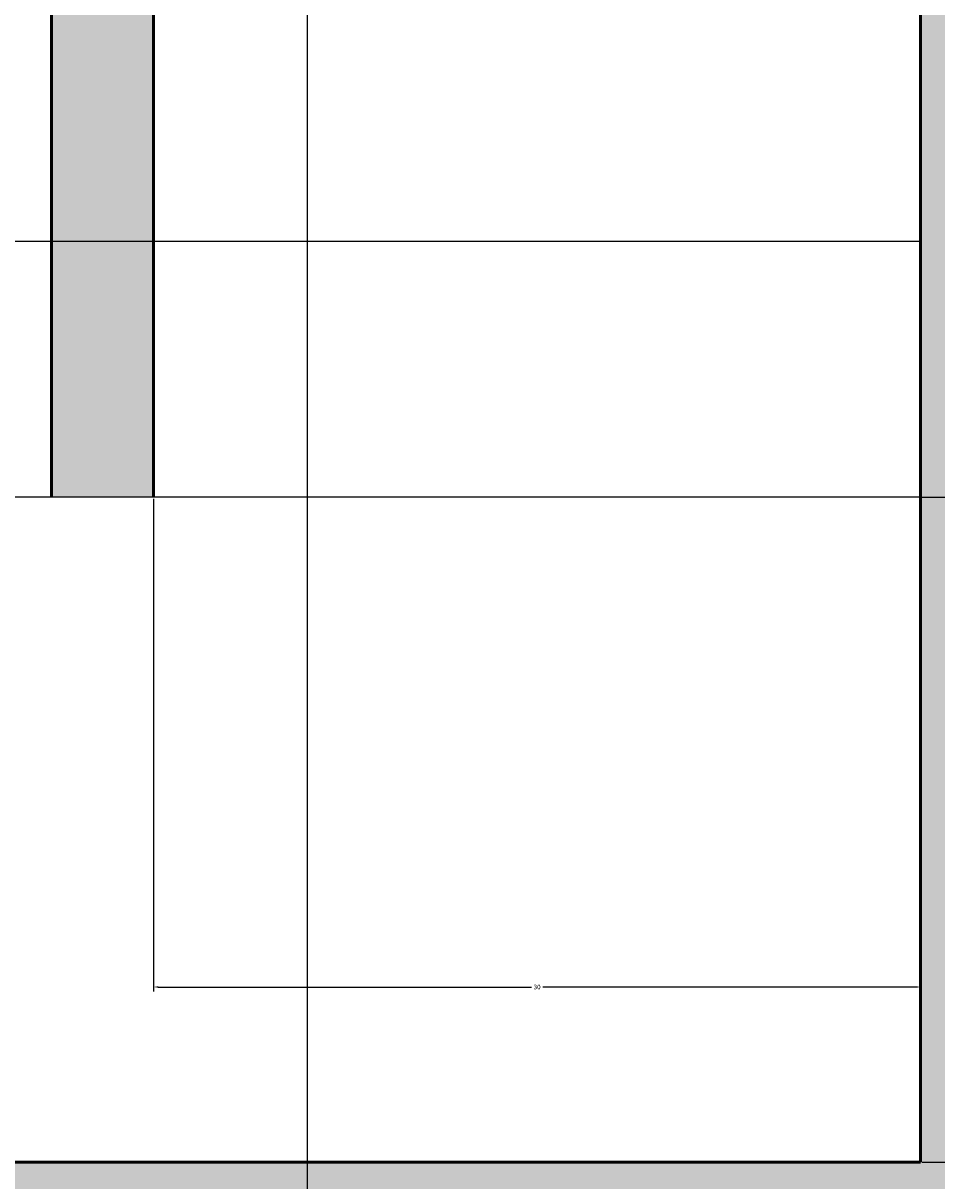
# Model space of a CAD drawing. Units: inches. Extents: x 2307 to 2544, y 2171 to 2540.
# Tile 11 of 52: x 2481 to 2516, y 2199 to 2244. Entities that reach past the tile are written whole.
import ezdxf

# ---------------------------------------------------------------- set-up
doc = ezdxf.new("R2010")
doc.units = ezdxf.units.IN
for name, color, linetype, lineweight in [('A-ANNO-DIMS', 2, 'Continuous', 18), ('A-FLOR-STRS', 7, 'Continuous', 25), ('A-WALL', 7, 'Continuous', 50)]:
    doc.layers.add(name, color=color, linetype=linetype, lineweight=lineweight)
doc.layers.add('A-WALL-PATT', color=18, linetype='Continuous', lineweight=13, true_color=0x000000)
doc.styles.get("Standard").update_dxf_attribs({"font": 'arial.ttf'})
doc.dimstyles.get("Standard").update_dxf_attribs({"dimtxt": 0.18, "dimasz": 0.18, "dimexe": 0.18, "dimexo": 0.0625, "dimgap": 0.09, "dimtad": 0, "dimtih": 1, "dimtoh": 1, "dimdec": 4, "dimzin": 0, "dimdsep": 46, "dimtxsty": 'Standard', "dimcen": 0.09, "dimadec": 0, "dimazin": 0, "dimtfac": 1, "dimtdec": 4, "dimtofl": 0, "dimtmove": 0, "dimatfit": 3, "dimfxl": 1, "dimtolj": 1, "dimtzin": 0, "dimarcsym": 0})

# ---------------------------------------------------------------- blocks, each defined once
blk = doc.blocks.new('*D54')
at = {"layer": 'A-ANNO-DIMS', "color": 0, "lineweight": -2, "transparency": 16777216}
for p, q in [((2461.696, 2435.447), (2461.696, 2171.18)), ((2491.696, 2435.447), (2491.696, 2171.18)), ((2461.876, 2171.36), (2476.477, 2171.36)), ((2491.516, 2171.36), (2476.914, 2171.36))]:
    blk.add_line(p, q, dxfattribs=at)
at = {"layer": 'A-ANNO-DIMS', "color": 0, "transparency": 16777216}
for points in [[(2461.876, 2171.39), (2461.876, 2171.33), (2461.696, 2171.36)], [(2491.516, 2171.39), (2491.516, 2171.33), (2491.696, 2171.36)]]:
    blk.add_solid(points, dxfattribs=at)
at = {"layer": 'Defpoints', "color": 0, "transparency": 16777216}
for p in [(2461.696, 2435.51), (2491.696, 2435.51), (2491.696, 2171.36)]:
    blk.add_point(p, dxfattribs=at)
at = {"layer": 'A-ANNO-DIMS', "color": 0, "transparency": 16777216, "insert": (2476.696, 2171.36), "char_height": 0.18, "attachment_point": 5}
blk.add_mtext('\\A1;30', dxfattribs=at)
blk = doc.blocks.new('*D55')
at = {"layer": 'A-ANNO-DIMS', "color": 0, "lineweight": -2, "transparency": 16777216}
for p, q in [((2485.696, 2225.447), (2485.696, 2206.18)), ((2515.696, 2225.447), (2515.696, 2206.18)), ((2485.876, 2206.36), (2500.477, 2206.36)), ((2515.516, 2206.36), (2500.914, 2206.36))]:
    blk.add_line(p, q, dxfattribs=at)
at = {"layer": 'A-ANNO-DIMS', "color": 0, "transparency": 16777216}
for points in [[(2485.876, 2206.39), (2485.876, 2206.33), (2485.696, 2206.36)], [(2515.516, 2206.39), (2515.516, 2206.33), (2515.696, 2206.36)]]:
    blk.add_solid(points, dxfattribs=at)
at = {"layer": 'Defpoints', "color": 0, "transparency": 16777216}
for p in [(2485.696, 2225.51), (2515.696, 2225.51), (2485.696, 2206.36)]:
    blk.add_point(p, dxfattribs=at)
at = {"layer": 'A-ANNO-DIMS', "color": 0, "transparency": 16777216, "insert": (2500.696, 2206.36), "char_height": 0.18, "attachment_point": 5}
blk.add_mtext('\\A1;30', dxfattribs=at)
blk = doc.blocks.new('*D56')
at = {"layer": 'A-ANNO-DIMS', "color": 0, "lineweight": -2, "transparency": 16777216}
for p, q in [((2515.758, 2285.51), (2544.026, 2285.51)), ((2543.846, 2285.33), (2543.846, 2255.691)), ((2543.846, 2225.69), (2543.846, 2255.328)), ((2515.758, 2225.51), (2544.026, 2225.51))]:
    blk.add_line(p, q, dxfattribs=at)
at = {"layer": 'A-ANNO-DIMS', "color": 0, "transparency": 16777216}
for points in [[(2543.816, 2285.33), (2543.876, 2285.33), (2543.846, 2285.51)], [(2543.816, 2225.69), (2543.876, 2225.69), (2543.846, 2225.51)]]:
    blk.add_solid(points, dxfattribs=at)
at = {"layer": 'Defpoints', "color": 0, "transparency": 16777216}
for p in [(2515.696, 2285.51), (2543.846, 2285.51), (2515.696, 2225.51)]:
    blk.add_point(p, dxfattribs=at)
at = {"layer": 'A-ANNO-DIMS', "color": 0, "transparency": 16777216, "insert": (2543.846, 2255.51), "char_height": 0.18, "attachment_point": 5}
blk.add_mtext('\\A1;60', dxfattribs=at)
blk = doc.blocks.new('*D58')
at = {"layer": 'A-ANNO-DIMS', "color": 0, "lineweight": -2, "transparency": 16777216}
for p, q in [((2485.633, 2235.51), (2466.366, 2235.51)), ((2466.546, 2235.33), (2466.546, 2230.691)), ((2466.546, 2225.69), (2466.546, 2230.328)), ((2485.633, 2225.51), (2466.366, 2225.51))]:
    blk.add_line(p, q, dxfattribs=at)
at = {"layer": 'A-ANNO-DIMS', "color": 0, "transparency": 16777216}
for points in [[(2466.516, 2235.33), (2466.576, 2235.33), (2466.546, 2235.51)], [(2466.516, 2225.69), (2466.576, 2225.69), (2466.546, 2225.51)]]:
    blk.add_solid(points, dxfattribs=at)
at = {"layer": 'Defpoints', "color": 0, "transparency": 16777216}
for p in [(2466.546, 2235.51), (2485.696, 2235.51), (2485.696, 2225.51)]:
    blk.add_point(p, dxfattribs=at)
at = {"layer": 'A-ANNO-DIMS', "color": 0, "transparency": 16777216, "insert": (2466.546, 2230.51), "char_height": 0.18, "attachment_point": 5}
blk.add_mtext('\\A1;10', dxfattribs=at)
blk = doc.blocks.new('*D60')
at = {"layer": 'A-ANNO-DIMS', "color": 0, "lineweight": -2, "transparency": 16777216}
for p, q in [((2515.758, 2225.51), (2544.026, 2225.51)), ((2543.846, 2225.33), (2543.846, 2212.691)), ((2543.846, 2199.69), (2543.846, 2212.328)), ((2515.758, 2199.51), (2544.026, 2199.51))]:
    blk.add_line(p, q, dxfattribs=at)
at = {"layer": 'A-ANNO-DIMS', "color": 0, "transparency": 16777216}
for points in [[(2543.816, 2225.33), (2543.876, 2225.33), (2543.846, 2225.51)], [(2543.816, 2199.69), (2543.876, 2199.69), (2543.846, 2199.51)]]:
    blk.add_solid(points, dxfattribs=at)
at = {"layer": 'Defpoints', "color": 0, "transparency": 16777216}
for p in [(2515.696, 2225.51), (2543.846, 2225.51), (2515.696, 2199.51)]:
    blk.add_point(p, dxfattribs=at)
at = {"layer": 'A-ANNO-DIMS', "color": 0, "transparency": 16777216, "insert": (2543.846, 2212.51), "char_height": 0.18, "attachment_point": 5}
blk.add_mtext('\\A1;26', dxfattribs=at)

msp = doc.modelspace()

# ---------------------------------------------------------------- hatches: boundary and pattern name
at = {"layer": 'A-WALL-PATT'}
h = msp.add_hatch(color=256, dxfattribs=at)
h.dxf.hatch_style = 1
h.paths.add_polyline_path([(2433.6935, 2199.5096), (2415.6423, 2199.5096), (2415.6423, 2190.5096), (2433.7832, 2190.5096)], flags=17)
h.paths.add_polyline_path([(2367.6423, 2199.5096), (2335.6958, 2199.5096), (2335.6958, 2307.3983), (2326.6958, 2307.3983), (2326.6958, 2190.5096), (2367.6423, 2190.5096)])
h.paths.add_polyline_path([(2524.6958, 2520.5096), (2496.7832, 2520.5096), (2496.7832, 2515.5149), (2472.7832, 2515.5149), (2472.7832, 2520.5096), (2415.4028, 2520.5096), (2415.4028, 2511.5096), (2451.6958, 2511.5096), (2451.6958, 2439.5096), (2451.6958, 2391.5096), (2445.6958, 2391.5096), (2445.6958, 2387.5096), (2455.6958, 2387.5096), (2455.6958, 2435.5096), (2461.6958, 2435.5096), (2461.6958, 2439.5096), (2455.6958, 2439.5096), (2455.6958, 2511.5096), (2515.6958, 2511.5096), (2515.6958, 2439.5096), (2491.6958, 2439.5096), (2491.6958, 2435.5096), (2515.6958, 2435.5096), (2515.6958, 2319.5096), (2451.6958, 2319.5096), (2451.6958, 2281.5096), (2481.6958, 2281.5096), (2481.6958, 2225.5096), (2485.6958, 2225.5096), (2485.6958, 2285.5096), (2455.6958, 2285.5096), (2455.6958, 2315.5096), (2515.6958, 2315.5096), (2515.6958, 2199.5096), (2469.6952, 2199.5096), (2469.785, 2190.5096), (2524.6958, 2190.5096)])

# ---------------------------------------------------------------- linework, layer by layer
at = {"layer": 'A-FLOR-STRS'}
for p, q in [((2515.6958, 2235.5096), (2485.6958, 2235.5096)), ((2515.6958, 2225.5096), (2481.6958, 2225.5096))]:
    msp.add_line(p, q, dxfattribs=at)
at = {"layer": 'A-WALL'}
for p, q in [((2515.6958, 2315.5096), (2515.6958, 2199.5096)), ((2485.6958, 2285.5096), (2485.6958, 2225.5096)), ((2481.6958, 2281.5096), (2481.6958, 2225.5096)), ((2515.6958, 2199.5096), (2469.6952, 2199.5096))]:
    msp.add_line(p, q, dxfattribs=at)

# ---------------------------------------------------------------- dimensions: what is measured, and where the dimension line sits
at = {"layer": 'A-ANNO-DIMS'}
dim = msp.add_linear_dim(base=(2491.6958, 2171.3596), p1=(2461.6958, 2435.5096), p2=(2491.6958, 2435.5096), dimstyle='Standard', override={"dimdec": 0, "dimlfac": 1, "dimrnd": 0, "dimzin": 0, "dimdsep": 46, "dimlunit": 2}, dxfattribs=at)
dim.commit()
dim.dimension.update_dxf_attribs({"geometry": '*D54', "text_midpoint": (2476.6958, 2171.3596)})
for base, p1, p2, angle, picture, middle in [((2543.8458, 2285.5096), (2515.6958, 2225.5096), (2515.6958, 2285.5096), 90, '*D56', (2543.8458, 2255.5096)), ((2466.5458, 2235.5096), (2485.6958, 2225.5096), (2485.6958, 2235.5096), 90, '*D58', (2466.5458, 2230.5096)), ((2485.6958, 2206.3596), (2515.6958, 2225.5096), (2485.6958, 2225.5096), 180, '*D55', (2500.6958, 2206.3596)), ((2543.8458, 2225.5096), (2515.6958, 2199.5096), (2515.6958, 2225.5096), 90, '*D60', (2543.8458, 2212.5096))]:
    dim = msp.add_linear_dim(base=base, p1=p1, p2=p2, angle=angle, dimstyle='Standard', override={"dimdec": 0, "dimlfac": 1, "dimrnd": 0, "dimzin": 0, "dimdsep": 46, "dimlunit": 2}, dxfattribs=at)
    dim.commit()
    dim.dimension.update_dxf_attribs({"geometry": picture, "text_midpoint": middle})

doc.saveas('drawing.dxf')
